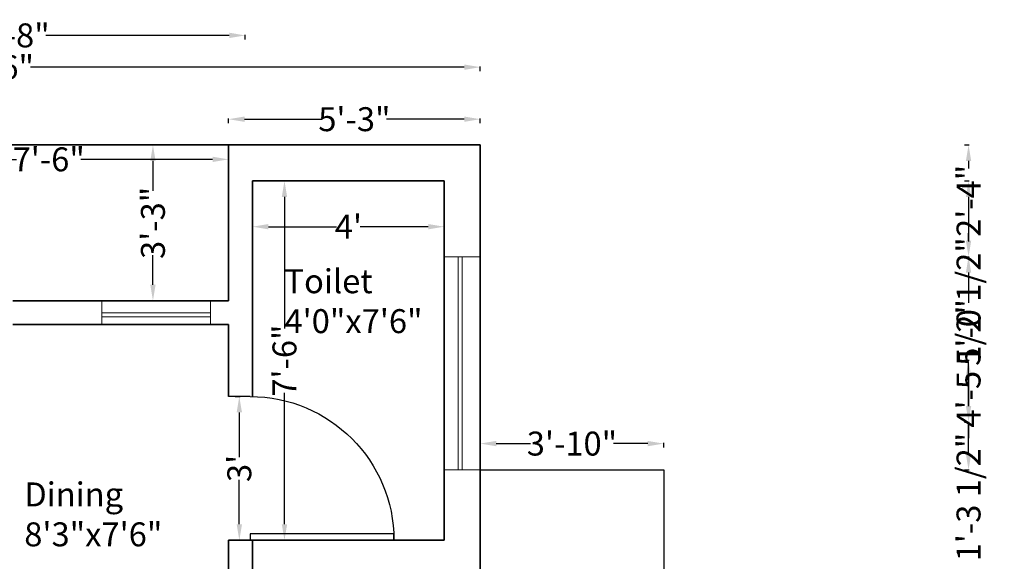
# Model space of a CAD drawing. Units: inches. Extents: x -81 to 380, y -521 to 79.
# Tile 5 of 5: x 134 to 380, y -76 to 60. Entities that reach past the tile are written whole.
import ezdxf

# ---------------------------------------------------------------- set-up
doc = ezdxf.new("R2010")
doc.units = ezdxf.units.IN
doc.header["$MEASUREMENT"] = 0
for name, color, linetype, lineweight in [('A-ANNO-DIMS', 2, 'Continuous', 18), ('A-AREA-IDEN', 5, 'Continuous', 25), ('A-FLOR-STRS', 6, 'Continuous', 25), ('A-GLAZ', 4, 'Continuous', 18), ('A-WALL', 249, 'Continuous', 35), ('door', 34, 'Continuous', 25)]:
    doc.layers.add(name, color=color, linetype=linetype, lineweight=lineweight)
doc.styles.get("Standard").update_dxf_attribs({"font": 'arial.ttf'})
doc.dimstyles.get("Standard").update_dxf_attribs({"dimtxt": 6, "dimasz": 4, "dimexe": 0.18, "dimexo": 0.0625, "dimgap": 0.09, "dimtad": 0, "dimdec": 0, "dimzin": 0, "dimdsep": 46, "dimlunit": 3, "dimtxsty": 'Standard', "dimcen": 0.09, "dimclrd": 6, "dimclre": 6, "dimclrt": 2, "dimadec": 0, "dimazin": 0, "dimtfac": 1, "dimtdec": 0, "dimtofl": 0, "dimtmove": 0, "dimatfit": 3, "dimfxl": 1, "dimfxlon": 1, "dimtolj": 1, "dimtzin": 0, "dimarcsym": 0})

# ---------------------------------------------------------------- blocks, each defined once
blk = doc.blocks.new('*U2')
for p, q in [((0, 0), (0, -6)), ((40, 0), (40, -6))]:
    blk.add_line(p, q)
blk.add_lwpolyline([(0, 0), (0, 40), (1.75, 40), (1.75, 0)], close=True)
blk.add_arc((0, 0), 40, 0, 90)
blk = doc.blocks.new('*D5')
at = {"layer": 'A-ANNO-DIMS', "color": 0, "lineweight": -2, "transparency": 16777216}
for p, q in [((3.31, 46.97), (3.31, 48.15)), ((7.31, 47.97), (115.86, 47.97)), ((245.31, 47.97), (136.76, 47.97)), ((249.31, 46.97), (249.31, 48.15))]:
    blk.add_line(p, q, dxfattribs=at)
at = {"layer": 'A-ANNO-DIMS', "color": 0, "transparency": 16777216}
for points in [[(7.31, 48.64), (7.31, 47.3), (3.31, 47.97)], [(245.31, 48.64), (245.31, 47.3), (249.31, 47.97)]]:
    blk.add_solid(points, dxfattribs=at)
at = {"layer": 'Defpoints', "color": 0, "transparency": 16777216}
for p in [(249.31, 47.97), (3.31, 28.48), (249.31, 28.48)]:
    blk.add_point(p, dxfattribs=at)
at = {"layer": 'A-ANNO-DIMS', "color": 0, "transparency": 16777216, "insert": (126.31, 47.97), "char_height": 6, "attachment_point": 5}
blk.add_mtext('\\A1;20\'-6"', dxfattribs=at)
blk = doc.blocks.new('*D9')
at = {"layer": 'A-ANNO-DIMS', "color": 0, "lineweight": -2, "transparency": 16777216}
for p, q in [((249.31, -47.31), (249.31, -46.13)), ((253.31, -46.31), (261.87, -46.31)), ((291.22, -46.31), (282.66, -46.31)), ((295.22, -47.31), (295.22, -46.13))]:
    blk.add_line(p, q, dxfattribs=at)
at = {"layer": 'A-ANNO-DIMS', "color": 0, "transparency": 16777216}
for points in [[(253.31, -45.64), (253.31, -46.98), (249.31, -46.31)], [(291.22, -45.64), (291.22, -46.98), (295.22, -46.31)]]:
    blk.add_solid(points, dxfattribs=at)
at = {"layer": 'Defpoints', "color": 0, "transparency": 16777216}
for p in [(295.22, -46.31), (249.31, -52.91), (295.22, -52.91)]:
    blk.add_point(p, dxfattribs=at)
at = {"layer": 'A-ANNO-DIMS', "color": 0, "transparency": 16777216, "insert": (272.26, -46.31), "char_height": 6, "attachment_point": 5}
blk.add_mtext('\\A1;3\'-10"', dxfattribs=at)
blk = doc.blocks.new('*D11')
at = {"layer": 'A-ANNO-DIMS', "color": 0, "lineweight": -2, "transparency": 16777216}
for p, q in [((186.31, 33.94), (186.31, 35.12)), ((190.31, 34.94), (209.75, 34.94)), ((245.31, 34.94), (225.88, 34.94)), ((249.31, 33.94), (249.31, 35.12))]:
    blk.add_line(p, q, dxfattribs=at)
at = {"layer": 'A-ANNO-DIMS', "color": 0, "transparency": 16777216}
for points in [[(190.31, 35.61), (190.31, 34.28), (186.31, 34.94)], [(245.31, 35.61), (245.31, 34.28), (249.31, 34.94)]]:
    blk.add_solid(points, dxfattribs=at)
at = {"layer": 'Defpoints', "color": 0, "transparency": 16777216}
for p in [(186.31, 34.94), (186.31, 28.48), (249.31, 28.48)]:
    blk.add_point(p, dxfattribs=at)
at = {"layer": 'A-ANNO-DIMS', "color": 0, "transparency": 16777216, "insert": (217.81, 34.94), "char_height": 6, "attachment_point": 5}
blk.add_mtext('\\A1;5\'-3"', dxfattribs=at)
blk = doc.blocks.new('*D15')
at = {"layer": 'A-ANNO-DIMS', "color": 0, "lineweight": -2, "transparency": 16777216}
for p, q in [((96.31, 24.88), (96.31, 25.06)), ((100.31, 24.88), (133.27, 24.88)), ((182.31, 24.88), (149.35, 24.88)), ((186.31, 24.88), (186.31, 25.06))]:
    blk.add_line(p, q, dxfattribs=at)
at = {"layer": 'A-ANNO-DIMS', "color": 0, "transparency": 16777216}
for points in [[(100.31, 25.55), (100.31, 24.21), (96.31, 24.88)], [(182.31, 25.55), (182.31, 24.21), (186.31, 24.88)]]:
    blk.add_solid(points, dxfattribs=at)
at = {"layer": 'Defpoints', "color": 0, "transparency": 16777216}
for p in [(96.31, 24.88), (186.31, 24.88), (186.31, 24.88)]:
    blk.add_point(p, dxfattribs=at)
at = {"layer": 'A-ANNO-DIMS', "color": 0, "transparency": 16777216, "insert": (141.31, 24.88), "char_height": 6, "attachment_point": 5}
blk.add_mtext('\\A1;7\'-6"', dxfattribs=at)
blk = doc.blocks.new('*D16')
at = {"layer": 'A-ANNO-DIMS', "color": 0, "lineweight": -2, "transparency": 16777216}
for p, q in [((167.39, 28.48), (167.57, 28.48)), ((167.39, 24.48), (167.39, 17.04)), ((167.39, -6.52), (167.39, 0.92)), ((167.39, -10.52), (167.57, -10.52))]:
    blk.add_line(p, q, dxfattribs=at)
at = {"layer": 'A-ANNO-DIMS', "color": 0, "transparency": 16777216}
for points in [[(166.72, 24.48), (168.06, 24.48), (167.39, 28.48)], [(166.72, -6.52), (168.06, -6.52), (167.39, -10.52)]]:
    blk.add_solid(points, dxfattribs=at)
at = {"layer": 'Defpoints', "color": 0, "transparency": 16777216}
for p in [(167.39, 28.48), (167.39, 28.48), (167.39, -10.52)]:
    blk.add_point(p, dxfattribs=at)
at = {"layer": 'A-ANNO-DIMS', "color": 0, "transparency": 16777216, "insert": (167.39, 8.98), "char_height": 6, "attachment_point": 5, "rotation": 90}
blk.add_mtext('\\A1;3\'-3"', dxfattribs=at)
blk = doc.blocks.new('*D17')
at = {"layer": 'A-ANNO-DIMS', "color": 0, "lineweight": -2, "transparency": 16777216}
for p, q in [((192.31, 8.02), (192.31, 8.2)), ((196.31, 8.02), (213.34, 8.02)), ((236.31, 8.02), (219.28, 8.02)), ((240.31, 8.02), (240.31, 8.2))]:
    blk.add_line(p, q, dxfattribs=at)
at = {"layer": 'A-ANNO-DIMS', "color": 0, "transparency": 16777216}
for points in [[(196.31, 8.68), (196.31, 7.35), (192.31, 8.02)], [(236.31, 8.68), (236.31, 7.35), (240.31, 8.02)]]:
    blk.add_solid(points, dxfattribs=at)
at = {"layer": 'Defpoints', "color": 0, "transparency": 16777216}
for p in [(192.31, 8.02), (240.31, 8.02), (240.31, 8.02)]:
    blk.add_point(p, dxfattribs=at)
at = {"layer": 'A-ANNO-DIMS', "color": 0, "transparency": 16777216, "insert": (216.31, 8.02), "char_height": 6, "attachment_point": 5}
blk.add_mtext("\\A1;4'", dxfattribs=at)
blk = doc.blocks.new('*D18')
at = {"layer": 'A-ANNO-DIMS', "color": 0, "lineweight": -2, "transparency": 16777216}
for p, q in [((201.31, 19.48), (200.13, 19.48)), ((200.31, 15.48), (200.31, -17.48)), ((200.31, -66.52), (200.31, -33.56)), ((201.31, -70.52), (200.13, -70.52))]:
    blk.add_line(p, q, dxfattribs=at)
at = {"layer": 'A-ANNO-DIMS', "color": 0, "transparency": 16777216}
for points in [[(199.64, 15.48), (200.98, 15.48), (200.31, 19.48)], [(199.64, -66.52), (200.98, -66.52), (200.31, -70.52)]]:
    blk.add_solid(points, dxfattribs=at)
at = {"layer": 'Defpoints', "color": 0, "transparency": 16777216}
for p in [(200.31, 19.48), (230.12, 19.48), (235.17, -70.52)]:
    blk.add_point(p, dxfattribs=at)
at = {"layer": 'A-ANNO-DIMS', "color": 0, "transparency": 16777216, "insert": (200.31, -25.52), "char_height": 6, "attachment_point": 5, "rotation": 90}
blk.add_mtext('\\A1;7\'-6"', dxfattribs=at)
blk = doc.blocks.new('*D26')
at = {"layer": 'A-ANNO-DIMS', "color": 0, "lineweight": -2, "transparency": 16777216}
for p, q in [((188.01, -34.52), (189.19, -34.52)), ((189.01, -38.52), (189.01, -49.67)), ((189.01, -66.52), (189.01, -55.37)), ((188.01, -70.52), (189.19, -70.52))]:
    blk.add_line(p, q, dxfattribs=at)
at = {"layer": 'A-ANNO-DIMS', "color": 0, "transparency": 16777216}
for points in [[(188.34, -38.52), (189.68, -38.52), (189.01, -34.52)], [(188.34, -66.52), (189.68, -66.52), (189.01, -70.52)]]:
    blk.add_solid(points, dxfattribs=at)
at = {"layer": 'Defpoints', "color": 0, "transparency": 16777216}
for p in [(186.31, -34.52), (186.31, -70.52), (189.01, -70.52)]:
    blk.add_point(p, dxfattribs=at)
at = {"layer": 'A-ANNO-DIMS', "color": 0, "transparency": 16777216, "insert": (189.01, -52.52), "char_height": 6, "attachment_point": 5, "rotation": 90}
blk.add_mtext("\\A1;3'", dxfattribs=at)
blk = doc.blocks.new('*D46')
at = {"layer": 'A-ANNO-DIMS', "color": 6, "lineweight": -2, "transparency": 16777216}
for p, q in [((74.55, 54.93), (74.55, 56.11)), ((78.55, 55.93), (124.45, 55.93)), ((186.48, 55.93), (140.58, 55.93)), ((190.48, 54.93), (190.48, 56.11))]:
    blk.add_line(p, q, dxfattribs=at)
at = {"layer": 'A-ANNO-DIMS', "color": 6, "transparency": 16777216}
for points in [[(78.55, 56.6), (78.55, 55.26), (74.55, 55.93)], [(186.48, 56.6), (186.48, 55.26), (190.48, 55.93)]]:
    blk.add_solid(points, dxfattribs=at)
at = {"layer": 'Defpoints', "color": 0, "transparency": 16777216}
for p in [(190.48, 55.93), (74.55, -489.67), (190.48, -489.67)]:
    blk.add_point(p, dxfattribs=at)
at = {"layer": 'A-ANNO-DIMS', "color": 2, "transparency": 16777216, "insert": (132.51, 55.93), "char_height": 6, "attachment_point": 5}
blk.add_mtext('\\A1;9\'-8"', dxfattribs=at)
blk = doc.blocks.new('*D54')
at = {"layer": 'A-ANNO-DIMS', "color": 6, "lineweight": -2, "transparency": 16777216}
for p, q in [((370.52, 19.48), (371.7, 19.48)), ((371.52, 15.48), (371.52, 4.34)), ((371.52, -36.92), (371.52, -25.77)), ((370.52, -40.92), (371.7, -40.92))]:
    blk.add_line(p, q, dxfattribs=at)
at = {"layer": 'A-ANNO-DIMS', "color": 6, "transparency": 16777216}
for points in [[(370.86, 15.48), (372.19, 15.48), (371.52, 19.48)], [(370.86, -36.92), (372.19, -36.92), (371.52, -40.92)]]:
    blk.add_solid(points, dxfattribs=at)
at = {"layer": 'Defpoints', "color": 0, "transparency": 16777216}
for p in [(90.31, 19.48), (90.31, -40.92), (371.52, -40.92)]:
    blk.add_point(p, dxfattribs=at)
at = {"layer": 'A-ANNO-DIMS', "color": 2, "transparency": 16777216, "insert": (371.52, -10.72), "char_height": 6, "attachment_point": 5, "rotation": 90}
blk.add_mtext('\\A1;5\'-0 1/2"', dxfattribs=at)
blk = doc.blocks.new('*D59')
at = {"layer": 'A-ANNO-DIMS', "color": 6, "lineweight": -2, "transparency": 16777216}
for p, q in [((370.52, -25.38), (371.7, -25.38)), ((371.52, -29.38), (371.52, -36.92)), ((370.52, -40.92), (371.7, -40.92)), ((371.52, -40.92), (371.52, -44.92))]:
    blk.add_line(p, q, dxfattribs=at)
at = {"layer": 'A-ANNO-DIMS', "color": 6, "transparency": 16777216}
for points in [[(370.86, -29.38), (372.19, -29.38), (371.52, -25.38)], [(370.86, -36.92), (372.19, -36.92), (371.52, -40.92)]]:
    blk.add_solid(points, dxfattribs=at)
at = {"layer": 'Defpoints', "color": 0, "transparency": 16777216}
for p in [(88.73, -25.38), (90.31, -40.92), (371.52, -40.92)]:
    blk.add_point(p, dxfattribs=at)
at = {"layer": 'A-ANNO-DIMS', "color": 2, "transparency": 16777216, "insert": (371.52, -59.69), "char_height": 6, "attachment_point": 5, "rotation": 90}
blk.add_mtext('\\A1;1\'-3 1/2"', dxfattribs=at)
blk = doc.blocks.new('*D67')
at = {"layer": 'A-ANNO-DIMS', "color": 6, "lineweight": -2, "transparency": 16777216}
for p, q in [((370.52, 0.51), (371.7, 0.51)), ((371.52, -3.49), (371.52, -11.02)), ((371.52, -48.91), (371.52, -41.38)), ((370.52, -52.91), (371.7, -52.91))]:
    blk.add_line(p, q, dxfattribs=at)
at = {"layer": 'A-ANNO-DIMS', "color": 6, "transparency": 16777216}
for points in [[(370.86, -3.49), (372.19, -3.49), (371.52, 0.51)], [(370.86, -48.91), (372.19, -48.91), (371.52, -52.91)]]:
    blk.add_solid(points, dxfattribs=at)
at = {"layer": 'Defpoints', "color": 0, "transparency": 16777216}
for p in [(249.31, 0.51), (371.52, 0.51), (249.31, -52.91)]:
    blk.add_point(p, dxfattribs=at)
at = {"layer": 'A-ANNO-DIMS', "color": 2, "transparency": 16777216, "insert": (371.52, -26.2), "char_height": 6, "attachment_point": 5, "rotation": 90}
blk.add_mtext('\\A1;4\'-5 1/2"', dxfattribs=at)
blk = doc.blocks.new('*D68')
at = {"layer": 'A-ANNO-DIMS', "color": 6, "lineweight": -2, "transparency": 16777216}
for p, q in [((370.52, 28.48), (371.7, 28.48)), ((371.52, 24.48), (371.52, 22.61)), ((371.52, 4.51), (371.52, 6.38)), ((370.52, 0.51), (371.7, 0.51))]:
    blk.add_line(p, q, dxfattribs=at)
at = {"layer": 'A-ANNO-DIMS', "color": 6, "transparency": 16777216}
for points in [[(370.86, 24.48), (372.19, 24.48), (371.52, 28.48)], [(370.86, 4.51), (372.19, 4.51), (371.52, 0.51)]]:
    blk.add_solid(points, dxfattribs=at)
at = {"layer": 'Defpoints', "color": 0, "transparency": 16777216}
for p in [(249.31, 28.48), (371.52, 28.48), (249.31, 0.51)]:
    blk.add_point(p, dxfattribs=at)
at = {"layer": 'A-ANNO-DIMS', "color": 2, "transparency": 16777216, "insert": (371.52, 14.5), "char_height": 6, "attachment_point": 5, "rotation": 90}
blk.add_mtext('\\A1;2\'-4"', dxfattribs=at)

msp = doc.modelspace()

# ---------------------------------------------------------------- linework, layer by layer
at = {"layer": 'A-FLOR-STRS'}
for p, q in [((249.31, -52.91), (295.22, -52.91)), ((295.22, -52.91), (295.22, -292.11))]:
    msp.add_line(p, q, dxfattribs=at)
at = {"layer": 'A-GLAZ'}
for p, q in [((240.31, 0.51), (249.31, 0.51)), ((243.81, -52.91), (243.81, 0.51)), ((244.81, -52.91), (244.81, 0.51)), ((154.58, -10.52), (154.58, -16.52)), ((181.8, -10.52), (181.8, -16.52)), ((181.8, -13.52), (154.58, -13.52)), ((181.8, -14.52), (154.58, -14.52)), ((240.31, -52.91), (249.31, -52.91))]:
    msp.add_line(p, q, dxfattribs=at)
at = {"layer": 'A-WALL'}
for p, q in [((3.31, 28.48), (249.31, 28.48)), ((186.31, 28.48), (186.31, -10.52)), ((249.31, 28.48), (249.31, -259.52)), ((192.31, 19.48), (192.31, -34.52)), ((192.31, 19.48), (240.31, 19.48)), ((240.31, 19.48), (240.31, -70.52)), ((132.31, -10.52), (186.31, -10.52)), ((132.31, -16.52), (186.31, -16.52)), ((186.31, -16.52), (186.31, -34.52)), ((186.31, -70.52), (240.31, -70.52)), ((186.31, -70.52), (186.31, -117.52)), ((192.31, -70.52), (192.31, -117.52))]:
    msp.add_line(p, q, dxfattribs=at)

# ---------------------------------------------------------------- block references
at = {"layer": 'door', "xscale": -0.9, "yscale": 0.9, "zscale": 0.9, "rotation": 270}
msp.add_blockref('*U2', (191.71, -70.52), dxfattribs=at)

# ---------------------------------------------------------------- texts
at = {"layer": 'A-AREA-IDEN', "char_height": 6, "attachment_point": 1}
for s, insert in [('Toilet\\P4\'0"x7\'6"', (200.31, -2.64)), ('Dining\\P8\'3"x7\'6"', (135.19, -56.04))]:
    msp.add_mtext_dynamic_manual_height_columns(s, width=81.6384, gutter_width=1, heights=[0], dxfattribs=dict(at, insert=insert))

# ---------------------------------------------------------------- dimensions: what is measured, and where the dimension line sits
at = {"layer": 'A-ANNO-DIMS'}
for base, p1, p2, override, picture, middle in [((190.48, 55.93), (74.55, -489.67), (190.48, -489.67), {"dimdec": 1, "dimlfac": 1, "dimrnd": 0, "dimzin": 1, "dimdsep": 46, "dimlunit": 4, "dimfrac": 2}, '*D46', (132.51, 55.93)), ((249.31, 47.97), (3.31, 28.48), (249.31, 28.48), {"dimclrd": 0, "dimclre": 0, "dimclrt": 0}, '*D5', (126.31, 47.97)), ((186.31, 34.94), (249.31, 28.48), (186.31, 28.48), {"dimclrd": 0, "dimclre": 0, "dimclrt": 0}, '*D11', (217.81, 34.94)), ((186.31, 24.88), (96.31, 24.88), (186.31, 24.88), {"dimclrd": 0, "dimclre": 0, "dimclrt": 0}, '*D15', (141.31, 24.88)), ((240.31, 8.02), (192.31, 8.02), (240.31, 8.02), {"dimclrd": 0, "dimclre": 0, "dimclrt": 0}, '*D17', (216.31, 8.02)), ((295.22, -46.31), (249.31, -52.91), (295.22, -52.91), {"dimclrd": 0, "dimclre": 0, "dimclrt": 0}, '*D9', (272.26, -46.31))]:
    dim = msp.add_linear_dim(base=base, p1=p1, p2=p2, dimstyle='Standard', override=override, dxfattribs=at)
    dim.commit()
    dim.dimension.update_dxf_attribs({"geometry": picture, "text_midpoint": middle})
for base, p1, p2, override, picture, middle in [((167.39, 28.48), (167.39, -10.52), (167.39, 28.48), {"dimclrd": 0, "dimclre": 0, "dimclrt": 0}, '*D16', (167.39, 8.98)), ((371.52, 28.48), (249.31, 0.51), (249.31, 28.48), {"dimdec": 1, "dimlfac": 1, "dimrnd": 0, "dimzin": 1, "dimdsep": 46, "dimlunit": 4, "dimfrac": 2}, '*D68', (371.52, 14.5)), ((371.52, -40.92), (90.31, 19.48), (90.31, -40.92), {"dimdec": 1, "dimlfac": 1, "dimrnd": 0, "dimzin": 1, "dimdsep": 46, "dimlunit": 4, "dimfrac": 2}, '*D54', (371.52, -10.72)), ((200.31, 19.48), (235.17, -70.52), (230.12, 19.48), {"dimclrd": 0, "dimclre": 0, "dimclrt": 0}, '*D18', (200.31, -25.52)), ((371.52, 0.51), (249.31, -52.91), (249.31, 0.51), {"dimdec": 1, "dimlfac": 1, "dimrnd": 0, "dimzin": 1, "dimdsep": 46, "dimlunit": 4, "dimfrac": 2}, '*D67', (371.52, -26.2)), ((371.52, -40.92), (88.73, -25.38), (90.31, -40.92), {"dimdec": 1, "dimlfac": 1, "dimrnd": 0, "dimzin": 1, "dimdsep": 46, "dimlunit": 4, "dimfrac": 2}, '*D59', (371.52, -59.69)), ((189.01, -70.52), (186.31, -34.52), (186.31, -70.52), {"dimclrd": 0, "dimclre": 0, "dimclrt": 0}, '*D26', (189.01, -52.52))]:
    dim = msp.add_linear_dim(base=base, p1=p1, p2=p2, angle=90, dimstyle='Standard', override=override, dxfattribs=at)
    dim.commit()
    dim.dimension.update_dxf_attribs({"geometry": picture, "text_midpoint": middle})

doc.saveas('drawing.dxf')
